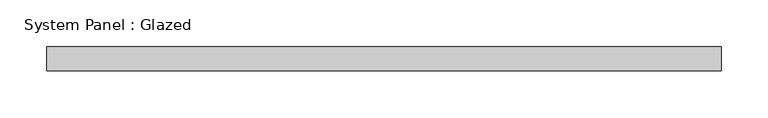
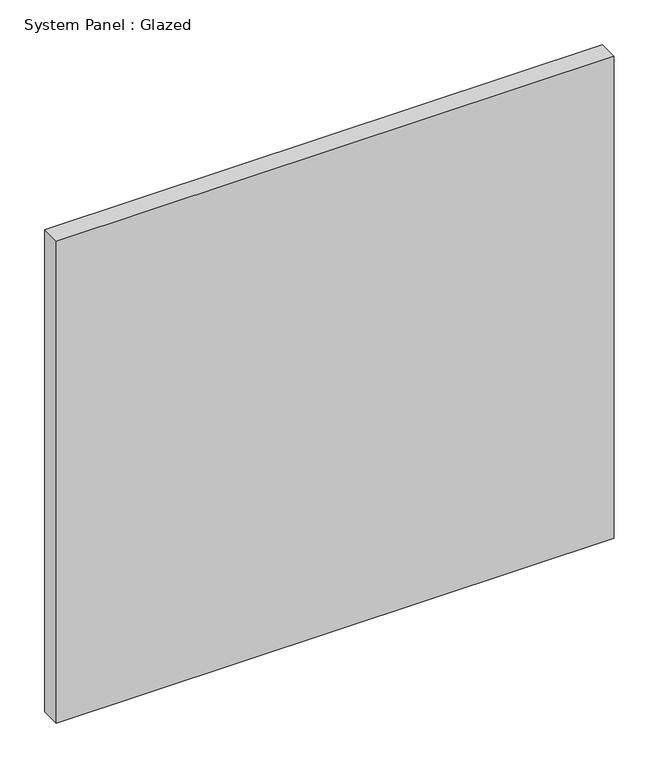
"""IFC4 building model written with IfcOpenShell, lengths in millimetres: plate geometry, System Panel : Glazed."""

from ifc_helpers import new_model, si_unit, origin, origin_with_axes, place, context, project, spatial, polyline, outline, extrude, source, transform, mapped, element, save


def system_panel_glazed_53cab8c3(model_context):
    return source(origin(), model_context, "Body", "SweptSolid", [
        extrude(outline(polyline([(358.775, 19.05), (-358.775, 19.05), (-358.775, 44.45), (358.775, 44.45), (358.775, 19.05)])), origin_with_axes(), (0.0, 0.0, 1.0), 655.366916),
    ])


if __name__ == "__main__":
    model = new_model("IFC4")
    model_context = context("Model", 3, world=origin())
    ifc_project = project(units=[si_unit("LENGTHUNIT", "METRE", prefix="MILLI")], contexts=[model_context])
    site = spatial("IfcSite", under=ifc_project)
    building = spatial("IfcBuilding", under=site)
    placement = place(None, origin())
    system_panel_glazed_shape = system_panel_glazed_53cab8c3(model_context)
    element("IfcPlate", 1, ObjectType="System Panel : Glazed", at=placement, inside=building, context=model_context, shape_type="MappedRepresentation", body=[
        mapped(system_panel_glazed_shape, transform((0.0, 0.0, 0.0), x_axis=(1.0, 0.0, 0.0), y_axis=(0.0, 1.0, 0.0), z_axis=(0.0, 0.0, 1.0))),
    ])
    save(model, "model.ifc")

# Revit data of these elements
# Type "System Panel : Glazed"
#   Construction Type Id = "GSP4R"
#   Analytic Construction = "1/8 in Pilkington single glazing"
#   Visual Light Transmittance = 0.9
#   Solar Heat Gain Coefficient = 0.86
#   Heat Transfer Coefficient (U) = 1.18115 BTU/(h·ft²·°F)
#   Define Thermal Properties by = 1
# Element 1 (IfcPlate, "System Panel : Glazed")
#   Materials on its faces: "Glass"
# Materials
#   "Glass": class "Glass", colour RGB 0 128 192, transparency 0.75, Description = "Soda Lime Glass", Cost = 0
